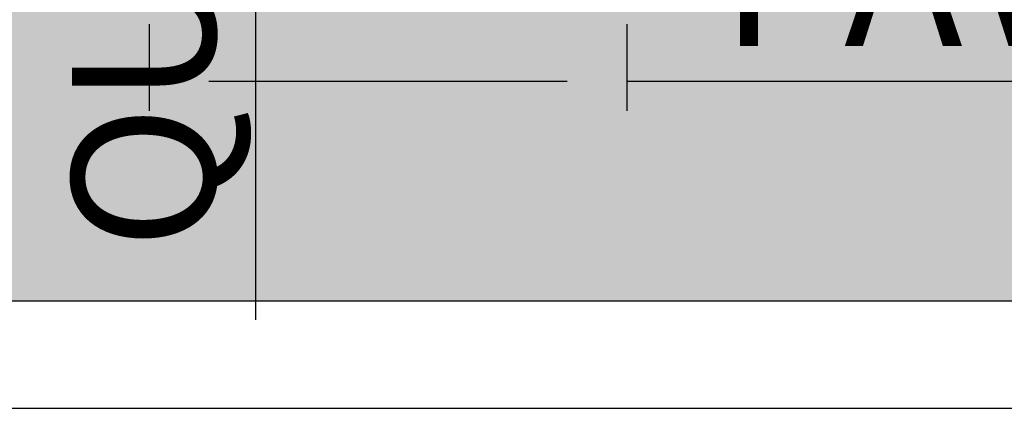
# Model space of a CAD drawing. Units: inches. Extents: x 459864 to 460310, y 324185 to 324787.
# Tile 45 of 112: x 460127 to 460169, y 324195 to 324211. Entities that reach past the tile are written whole.
import ezdxf

# ---------------------------------------------------------------- set-up
doc = ezdxf.new("R2010")
doc.units = ezdxf.units.IN
for name, color, linetype, lineweight in [('A-ANNO-DIMS', 2, 'Continuous', 18), ('C-PROP', 7, 'Continuous', 30), ('L-SITE-PATT', 252, 'Continuous', 13)]:
    doc.layers.add(name, color=color, linetype=linetype, lineweight=lineweight)
doc.styles.get("Standard").update_dxf_attribs({"font": 'arial.ttf'})
doc.dimstyles.new('ISO-25', dxfattribs={"dimtxt": 6, "dimasz": 2.5, "dimexe": 1.25, "dimexo": 0.625, "dimtad": 1, "dimdec": 1, "dimlunit": 3, "dimtxsty": 'Standard', "dimcen": 2.5, "dimadec": 0, "dimazin": 0, "dimtfac": 1, "dimtdec": 1, "dimtmove": 0, "dimatfit": 3, "dimfxl": 1, "dimarcsym": 0})

# ---------------------------------------------------------------- blocks, each defined once
blk = doc.blocks.new('*D28')
at = {"layer": 'A-ANNO-DIMS', "color": 0, "lineweight": -2, "transparency": 16777216}
for p, q in [((460148.65, 324370.7), (460136.025, 324370.7)), ((460137.275, 324368.2), (460137.275, 324293.2)), ((460148.65, 324290.7), (460136.025, 324290.7)), ((460137.275, 324290.7), (460137.275, 324198.69))]:
    blk.add_line(p, q, dxfattribs=at)
at = {"layer": 'A-ANNO-DIMS', "color": 0, "transparency": 16777216}
for points in [[(460136.858, 324368.2), (460137.692, 324368.2), (460137.275, 324370.7)], [(460136.858, 324293.2), (460137.692, 324293.2), (460137.275, 324290.7)]]:
    blk.add_solid(points, dxfattribs=at)
at = {"layer": 'Defpoints', "color": 0, "transparency": 16777216}
for p in [(460149.275, 324370.7), (460137.275, 324290.7), (460149.275, 324290.7)]:
    blk.add_point(p, dxfattribs=at)
at = {"layer": 'A-ANNO-DIMS', "color": 0, "transparency": 16777216, "insert": (460133.363, 324243.445), "char_height": 6, "attachment_point": 5, "rotation": 90}
blk.add_mtext('QUEEN BED 6\'-8" TYP.', dxfattribs=at)
blk = doc.blocks.new('*D34')
at = {"layer": 'A-ANNO-DIMS', "color": 0, "lineweight": -2, "transparency": 16777216}
for p, q in [((460132.814, 324211.063), (460132.814, 324207.434)), ((460152.838, 324211.063), (460152.838, 324207.434)), ((460135.314, 324208.684), (460150.338, 324208.684)), ((460152.838, 324208.684), (460202.984, 324208.684))]:
    blk.add_line(p, q, dxfattribs=at)
at = {"layer": 'A-ANNO-DIMS', "color": 0, "transparency": 16777216}
for points in [[(460135.314, 324209.101), (460135.314, 324208.268), (460132.814, 324208.684)], [(460150.338, 324209.101), (460150.338, 324208.268), (460152.838, 324208.684)]]:
    blk.add_solid(points, dxfattribs=at)
at = {"layer": 'Defpoints', "color": 0, "transparency": 16777216}
for p in [(460132.814, 324211.688), (460152.838, 324211.688), (460152.838, 324208.684)]:
    blk.add_point(p, dxfattribs=at)
at = {"layer": 'A-ANNO-DIMS', "color": 0, "transparency": 16777216, "insert": (460179.161, 324212.373), "char_height": 6, "attachment_point": 5}
blk.add_mtext('PAVER 1\'-8"', dxfattribs=at)

msp = doc.modelspace()

# ---------------------------------------------------------------- hatches: boundary and pattern name
at = {"layer": 'L-SITE-PATT'}
h = msp.add_hatch(dxfattribs=at)
h.set_pattern_fill('DOTS', color=256)
h.paths.add_polyline_path([(460269.804, 324283.483), (460247.115, 324283.483), (460121.929, 324283.483), (460121.929, 324252.473), (460117.429, 324252.473), (460110.124, 324252.473), (460110.124, 324243.287), (460080.83, 324243.287), (460080.83, 324252.473), (460061.115, 324252.473), (460061.115, 324251.882), (460077.909, 324251.882), (460077.909, 324199.483), (460080.83, 324199.483), (460080.83, 324207.553), (460110.124, 324207.553), (460110.124, 324199.483), (460110.813, 324199.483), (460262.115, 324199.483), (460269.804, 324199.483)], flags=17)
edge = h.paths.add_edge_path(flags=0)
edge.add_ellipse((460222.59, 324263.813), major_axis=(-8.485, 8.485), ratio=1, start_angle=405, end_angle=495, ccw=False)
edge.add_line((460214.821, 324254.66), (460214.832, 324254.666))
edge.add_ellipse((460222.59, 324263.813), major_axis=(-8.485, 8.485), ratio=1, start_angle=405, end_angle=495, ccw=False)
edge.add_line((460210.759, 324261.781), (460210.768, 324261.787))
edge.add_ellipse((460222.59, 324263.813), major_axis=(-8.485, 8.485), ratio=1, start_angle=405, end_angle=495, ccw=False)
edge.add_ellipse((460222.59, 324263.813), major_axis=(-8.485, 8.485), ratio=1, start_angle=392.754, end_angle=405, ccw=False)
edge.add_ellipse((460222.59, 324263.813), major_axis=(-8.485, 8.485), ratio=1, start_angle=380.9347, end_angle=392.754, ccw=False)
edge.add_line((460211.337, 324267.985), (460211.34, 324267.985))
edge.add_ellipse((460222.59, 324263.813), major_axis=(-8.485, 8.485), ratio=1, start_angle=380.9347, end_angle=392.754, ccw=False)
edge.add_ellipse((460222.59, 324263.813), major_axis=(-8.485, 8.485), ratio=1, start_angle=347.9015, end_angle=380.9347, ccw=False)
edge.add_ellipse((460222.59, 324263.813), major_axis=(-8.485, 8.485), ratio=1, start_angle=327.0619, end_angle=347.9015, ccw=False)
edge.add_ellipse((460222.59, 324263.813), major_axis=(-8.485, 8.485), ratio=1, start_angle=278.3246, end_angle=327.0619, ccw=False)
edge.add_line((460225.158, 324275.536), (460225.158, 324275.535))
edge.add_ellipse((460222.59, 324263.813), major_axis=(-8.485, 8.485), ratio=1, start_angle=278.3246, end_angle=327.0619, ccw=False)
edge.add_ellipse((460222.59, 324263.813), major_axis=(-8.485, 8.485), ratio=1, start_angle=260.6436, end_angle=278.3246, ccw=False)
edge.add_ellipse((460222.59, 324263.813), major_axis=(-8.485, 8.485), ratio=1, start_angle=225, end_angle=260.6436, ccw=False)
edge.add_line((460234.509, 324265.243), (460234.501, 324265.239))
edge.add_ellipse((460222.59, 324263.813), major_axis=(-8.485, 8.485), ratio=1, start_angle=225, end_angle=260.6436, ccw=False)
edge.add_ellipse((460222.59, 324263.813), major_axis=(-8.485, 8.485), ratio=1, start_angle=495, end_angle=585, ccw=False)
edge.add_line((460234.437, 324261.861), (460234.424, 324261.858))
edge.add_ellipse((460222.59, 324263.813), major_axis=(-8.485, 8.485), ratio=1, start_angle=495, end_angle=585, ccw=False)
edge.add_line((460227.95, 324253.067), (460227.946, 324253.083))
edge.add_ellipse((460222.59, 324263.813), major_axis=(-8.485, 8.485), ratio=1, start_angle=495, end_angle=585, ccw=False)
edge.add_line((460226.223, 324252.369), (460226.211, 324252.38))
edge.add_ellipse((460222.59, 324263.813), major_axis=(-8.485, 8.485), ratio=1, start_angle=495, end_angle=585, ccw=False)
h.paths.add_polyline_path([(460219.651, 324254.347), (460218.461, 324253.545), (460218.275, 324254.789), (460219.642, 324256.542), (460219.625, 324260.848), (460216.11, 324257.333), (460214.35, 324256.978), (460215.416, 324259.356), (460212.524, 324258.496), (460213.137, 324259.93), (460218.507, 324263.813), (460222.59, 324263.813), (460222.59, 324267.807), (460218.176, 324272.212), (460219.026, 324274.639), (460222.59, 324272.811), (460222.59, 324275.423), (460223.057, 324274.825), (460222.675, 324273.492), (460225.912, 324267.135), (460219.625, 324260.848)], flags=0)
edge = h.paths.add_edge_path(flags=0)
edge.add_ellipse((460194.576, 324264.046), major_axis=(-8.485, 8.485), ratio=1, start_angle=495, end_angle=585, ccw=False)
edge.add_line((460199.936, 324253.3), (460199.932, 324253.316))
edge.add_ellipse((460194.576, 324264.046), major_axis=(-8.485, 8.485), ratio=1, start_angle=495, end_angle=585, ccw=False)
edge.add_line((460198.208, 324252.603), (460198.196, 324252.613))
edge.add_ellipse((460194.576, 324264.046), major_axis=(-8.485, 8.485), ratio=1, start_angle=495, end_angle=585, ccw=False)
edge.add_ellipse((460194.576, 324264.046), major_axis=(-8.485, 8.485), ratio=1, start_angle=405, end_angle=495, ccw=False)
edge.add_line((460186.806, 324254.893), (460186.817, 324254.899))
edge.add_ellipse((460194.576, 324264.046), major_axis=(-8.485, 8.485), ratio=1, start_angle=405, end_angle=495, ccw=False)
edge.add_line((460182.744, 324262.014), (460182.753, 324262.02))
edge.add_ellipse((460194.576, 324264.046), major_axis=(-8.485, 8.485), ratio=1, start_angle=405, end_angle=495, ccw=False)
edge.add_ellipse((460194.576, 324264.046), major_axis=(-8.485, 8.485), ratio=1, start_angle=392.754, end_angle=405, ccw=False)
edge.add_ellipse((460194.576, 324264.046), major_axis=(-8.485, 8.485), ratio=1, start_angle=380.9347, end_angle=392.754, ccw=False)
edge.add_line((460183.323, 324268.218), (460183.326, 324268.218))
edge.add_ellipse((460194.576, 324264.046), major_axis=(-8.485, 8.485), ratio=1, start_angle=380.9347, end_angle=392.754, ccw=False)
edge.add_ellipse((460194.576, 324264.046), major_axis=(-8.485, 8.485), ratio=1, start_angle=347.9015, end_angle=380.9347, ccw=False)
edge.add_ellipse((460194.576, 324264.046), major_axis=(-8.485, 8.485), ratio=1, start_angle=327.0619, end_angle=347.9015, ccw=False)
edge.add_ellipse((460194.576, 324264.046), major_axis=(-8.485, 8.485), ratio=1, start_angle=278.3246, end_angle=327.0619, ccw=False)
edge.add_line((460197.144, 324275.769), (460197.143, 324275.768))
edge.add_ellipse((460194.576, 324264.046), major_axis=(-8.485, 8.485), ratio=1, start_angle=278.3246, end_angle=327.0619, ccw=False)
edge.add_ellipse((460194.576, 324264.046), major_axis=(-8.485, 8.485), ratio=1, start_angle=260.6436, end_angle=278.3246, ccw=False)
edge.add_ellipse((460194.576, 324264.046), major_axis=(-8.485, 8.485), ratio=1, start_angle=225, end_angle=260.6436, ccw=False)
edge.add_line((460206.494, 324265.476), (460206.487, 324265.473))
edge.add_ellipse((460194.576, 324264.046), major_axis=(-8.485, 8.485), ratio=1, start_angle=225, end_angle=260.6436, ccw=False)
edge.add_ellipse((460194.576, 324264.046), major_axis=(-8.485, 8.485), ratio=1, start_angle=495, end_angle=585, ccw=False)
edge.add_line((460206.422, 324262.094), (460206.409, 324262.091))
h.paths.add_polyline_path([(460191.61, 324261.081), (460191.637, 324254.58), (460190.447, 324253.778), (460190.261, 324255.023), (460191.628, 324256.775), (460191.61, 324261.081), (460188.096, 324257.566), (460186.335, 324257.211), (460187.402, 324259.589), (460184.509, 324258.729), (460185.123, 324260.163), (460190.493, 324264.046), (460194.576, 324264.046), (460194.576, 324268.04), (460190.161, 324272.446), (460191.011, 324274.872), (460194.576, 324273.044), (460194.576, 324275.657), (460195.043, 324275.058), (460194.661, 324273.725), (460197.897, 324267.368)], flags=0)
edge = h.paths.add_edge_path(flags=0)
edge.add_ellipse((460252.912, 324263.578), major_axis=(-8.485, 8.485), ratio=1, start_angle=405, end_angle=495, ccw=False)
edge.add_line((460241.081, 324261.545), (460241.089, 324261.551))
edge.add_ellipse((460252.912, 324263.578), major_axis=(-8.485, 8.485), ratio=1, start_angle=405, end_angle=495, ccw=False)
edge.add_ellipse((460252.912, 324263.578), major_axis=(-8.485, 8.485), ratio=1, start_angle=392.754, end_angle=405, ccw=False)
edge.add_ellipse((460252.912, 324263.578), major_axis=(-8.485, 8.485), ratio=1, start_angle=380.9347, end_angle=392.754, ccw=False)
edge.add_line((460241.659, 324267.749), (460241.662, 324267.749))
edge.add_ellipse((460252.912, 324263.578), major_axis=(-8.485, 8.485), ratio=1, start_angle=380.9347, end_angle=392.754, ccw=False)
edge.add_ellipse((460252.912, 324263.578), major_axis=(-8.485, 8.485), ratio=1, start_angle=347.9015, end_angle=380.9347, ccw=False)
edge.add_ellipse((460252.912, 324263.578), major_axis=(-8.485, 8.485), ratio=1, start_angle=327.0619, end_angle=347.9015, ccw=False)
edge.add_ellipse((460252.912, 324263.578), major_axis=(-8.485, 8.485), ratio=1, start_angle=278.3246, end_angle=327.0619, ccw=False)
edge.add_line((460255.48, 324275.3), (460255.479, 324275.299))
edge.add_ellipse((460252.912, 324263.578), major_axis=(-8.485, 8.485), ratio=1, start_angle=278.3246, end_angle=327.0619, ccw=False)
edge.add_ellipse((460252.912, 324263.578), major_axis=(-8.485, 8.485), ratio=1, start_angle=260.6436, end_angle=278.3246, ccw=False)
edge.add_ellipse((460252.912, 324263.578), major_axis=(-8.485, 8.485), ratio=1, start_angle=225, end_angle=260.6436, ccw=False)
edge.add_line((460264.83, 324265.007), (460264.823, 324265.004))
edge.add_ellipse((460252.912, 324263.578), major_axis=(-8.485, 8.485), ratio=1, start_angle=225, end_angle=260.6436, ccw=False)
edge.add_ellipse((460252.912, 324263.578), major_axis=(-8.485, 8.485), ratio=1, start_angle=495, end_angle=585, ccw=False)
edge.add_line((460264.758, 324261.626), (460264.745, 324261.622))
edge.add_ellipse((460252.912, 324263.578), major_axis=(-8.485, 8.485), ratio=1, start_angle=495, end_angle=585, ccw=False)
edge.add_line((460258.272, 324252.832), (460258.268, 324252.848))
edge.add_ellipse((460252.912, 324263.578), major_axis=(-8.485, 8.485), ratio=1, start_angle=495, end_angle=585, ccw=False)
edge.add_line((460256.545, 324252.134), (460256.533, 324252.144))
edge.add_ellipse((460252.912, 324263.578), major_axis=(-8.485, 8.485), ratio=1, start_angle=495, end_angle=585, ccw=False)
edge.add_ellipse((460252.912, 324263.578), major_axis=(-8.485, 8.485), ratio=1, start_angle=405, end_angle=495, ccw=False)
edge.add_line((460245.143, 324254.424), (460245.153, 324254.43))
h.paths.add_polyline_path([(460244.672, 324256.742), (460245.738, 324259.12), (460242.846, 324258.26), (460243.459, 324259.694), (460248.829, 324263.578), (460252.912, 324263.578), (460252.912, 324267.571), (460248.497, 324271.977), (460249.348, 324274.403), (460252.912, 324272.576), (460252.912, 324275.188), (460253.379, 324274.589), (460252.997, 324273.257), (460256.233, 324266.899), (460249.946, 324260.612), (460249.973, 324254.111), (460248.783, 324253.309), (460248.597, 324254.554), (460249.964, 324256.306), (460249.946, 324260.612), (460246.432, 324257.097)], flags=0)
edge = h.paths.add_edge_path(flags=0)
edge.add_ellipse((460167.439, 324262.833), major_axis=(-8.485, 8.485), ratio=1, start_angle=495, end_angle=585, ccw=False)
edge.add_line((460172.799, 324252.087), (460172.795, 324252.103))
edge.add_ellipse((460167.439, 324262.833), major_axis=(-8.485, 8.485), ratio=1, start_angle=495, end_angle=585, ccw=False)
edge.add_line((460171.071, 324251.389), (460171.059, 324251.399))
edge.add_ellipse((460167.439, 324262.833), major_axis=(-8.485, 8.485), ratio=1, start_angle=495, end_angle=585, ccw=False)
edge.add_ellipse((460167.439, 324262.833), major_axis=(-8.485, 8.485), ratio=1, start_angle=405, end_angle=495, ccw=False)
edge.add_line((460159.669, 324253.679), (460159.68, 324253.685))
edge.add_ellipse((460167.439, 324262.833), major_axis=(-8.485, 8.485), ratio=1, start_angle=405, end_angle=495, ccw=False)
edge.add_line((460155.607, 324260.8), (460155.616, 324260.806))
edge.add_ellipse((460167.439, 324262.833), major_axis=(-8.485, 8.485), ratio=1, start_angle=405, end_angle=495, ccw=False)
edge.add_ellipse((460167.439, 324262.833), major_axis=(-8.485, 8.485), ratio=1, start_angle=392.754, end_angle=405, ccw=False)
edge.add_ellipse((460167.439, 324262.833), major_axis=(-8.485, 8.485), ratio=1, start_angle=380.9347, end_angle=392.754, ccw=False)
edge.add_line((460156.185, 324267.005), (460156.189, 324267.005))
edge.add_ellipse((460167.439, 324262.833), major_axis=(-8.485, 8.485), ratio=1, start_angle=380.9347, end_angle=392.754, ccw=False)
edge.add_ellipse((460167.439, 324262.833), major_axis=(-8.485, 8.485), ratio=1, start_angle=347.9015, end_angle=380.9347, ccw=False)
edge.add_ellipse((460167.439, 324262.833), major_axis=(-8.485, 8.485), ratio=1, start_angle=327.0619, end_angle=347.9015, ccw=False)
edge.add_ellipse((460167.439, 324262.833), major_axis=(-8.485, 8.485), ratio=1, start_angle=278.3246, end_angle=327.0619, ccw=False)
edge.add_line((460170.007, 324274.556), (460170.006, 324274.554))
edge.add_ellipse((460167.439, 324262.833), major_axis=(-8.485, 8.485), ratio=1, start_angle=278.3246, end_angle=327.0619, ccw=False)
edge.add_ellipse((460167.439, 324262.833), major_axis=(-8.485, 8.485), ratio=1, start_angle=260.6436, end_angle=278.3246, ccw=False)
edge.add_ellipse((460167.439, 324262.833), major_axis=(-8.485, 8.485), ratio=1, start_angle=225, end_angle=260.6436, ccw=False)
edge.add_line((460179.357, 324264.262), (460179.35, 324264.259))
edge.add_ellipse((460167.439, 324262.833), major_axis=(-8.485, 8.485), ratio=1, start_angle=225, end_angle=260.6436, ccw=False)
edge.add_ellipse((460167.439, 324262.833), major_axis=(-8.485, 8.485), ratio=1, start_angle=495, end_angle=585, ccw=False)
edge.add_line((460179.285, 324260.881), (460179.272, 324260.877))
h.paths.add_polyline_path([(460164.473, 324259.867), (460164.5, 324253.366), (460163.31, 324252.565), (460163.124, 324253.809), (460164.491, 324255.561), (460164.473, 324259.867), (460160.958, 324256.353), (460159.198, 324255.998), (460160.265, 324258.375), (460157.372, 324257.515), (460157.986, 324258.949), (460163.356, 324262.833), (460167.439, 324262.833), (460167.439, 324266.826), (460163.024, 324271.232), (460163.874, 324273.659), (460167.439, 324271.831), (460167.439, 324274.443), (460167.905, 324273.844), (460167.524, 324272.512), (460170.76, 324266.154)], flags=0)
edge = h.paths.add_edge_path(flags=0)
edge.add_ellipse((460140.758, 324262.37), major_axis=(-8.485, 8.485), ratio=1, start_angle=495, end_angle=585, ccw=False)
edge.add_line((460146.118, 324251.624), (460146.114, 324251.639))
edge.add_ellipse((460140.758, 324262.37), major_axis=(-8.485, 8.485), ratio=1, start_angle=495, end_angle=585, ccw=False)
edge.add_line((460144.391, 324250.926), (460144.379, 324250.936))
edge.add_ellipse((460140.758, 324262.37), major_axis=(-8.485, 8.485), ratio=1, start_angle=495, end_angle=585, ccw=False)
edge.add_ellipse((460140.758, 324262.37), major_axis=(-8.485, 8.485), ratio=1, start_angle=405, end_angle=495, ccw=False)
edge.add_line((460132.989, 324253.216), (460132.999, 324253.222))
edge.add_ellipse((460140.758, 324262.37), major_axis=(-8.485, 8.485), ratio=1, start_angle=405, end_angle=495, ccw=False)
edge.add_line((460128.927, 324260.337), (460128.935, 324260.343))
edge.add_ellipse((460140.758, 324262.37), major_axis=(-8.485, 8.485), ratio=1, start_angle=405, end_angle=495, ccw=False)
edge.add_ellipse((460140.758, 324262.37), major_axis=(-8.485, 8.485), ratio=1, start_angle=392.754, end_angle=405, ccw=False)
edge.add_ellipse((460140.758, 324262.37), major_axis=(-8.485, 8.485), ratio=1, start_angle=380.9347, end_angle=392.754, ccw=False)
edge.add_line((460129.505, 324266.541), (460129.508, 324266.541))
edge.add_ellipse((460140.758, 324262.37), major_axis=(-8.485, 8.485), ratio=1, start_angle=380.9347, end_angle=392.754, ccw=False)
edge.add_ellipse((460140.758, 324262.37), major_axis=(-8.485, 8.485), ratio=1, start_angle=347.9015, end_angle=380.9347, ccw=False)
edge.add_ellipse((460140.758, 324262.37), major_axis=(-8.485, 8.485), ratio=1, start_angle=327.0619, end_angle=347.9015, ccw=False)
edge.add_ellipse((460140.758, 324262.37), major_axis=(-8.485, 8.485), ratio=1, start_angle=278.3246, end_angle=327.0619, ccw=False)
edge.add_line((460143.326, 324274.092), (460143.325, 324274.091))
edge.add_ellipse((460140.758, 324262.37), major_axis=(-8.485, 8.485), ratio=1, start_angle=278.3246, end_angle=327.0619, ccw=False)
edge.add_ellipse((460140.758, 324262.37), major_axis=(-8.485, 8.485), ratio=1, start_angle=260.6436, end_angle=278.3246, ccw=False)
edge.add_ellipse((460140.758, 324262.37), major_axis=(-8.485, 8.485), ratio=1, start_angle=225, end_angle=260.6436, ccw=False)
edge.add_line((460152.677, 324263.799), (460152.669, 324263.796))
edge.add_ellipse((460140.758, 324262.37), major_axis=(-8.485, 8.485), ratio=1, start_angle=225, end_angle=260.6436, ccw=False)
edge.add_ellipse((460140.758, 324262.37), major_axis=(-8.485, 8.485), ratio=1, start_angle=495, end_angle=585, ccw=False)
edge.add_line((460152.604, 324260.418), (460152.592, 324260.414))
h.paths.add_polyline_path([(460137.792, 324259.404), (460137.819, 324252.903), (460136.629, 324252.101), (460136.443, 324253.346), (460137.81, 324255.098), (460137.792, 324259.404), (460134.278, 324255.889), (460132.518, 324255.534), (460133.584, 324257.912), (460130.692, 324257.052), (460131.305, 324258.486), (460136.675, 324262.37), (460140.758, 324262.37), (460140.758, 324266.363), (460136.343, 324270.769), (460137.194, 324273.195), (460140.758, 324271.367), (460140.758, 324273.98), (460141.225, 324273.381), (460140.843, 324272.049), (460144.079, 324265.691)], flags=0)
h.paths.add_polyline_path([(460110.124, 324227.414), (460080.83, 324227.414), (460080.83, 324235.484), (460110.124, 324235.484)], flags=16)
h.paths.add_polyline_path([(460110.124, 324220.797), (460110.124, 324212.727), (460080.83, 324212.727), (460080.83, 324220.797)], flags=16)
h.paths.add_polyline_path([(460269.804, 324283.483), (460247.115, 324283.483), (460121.929, 324283.483), (460121.929, 324252.473), (460117.429, 324252.473), (460110.124, 324252.473), (460110.124, 324243.287), (460080.83, 324243.287), (460080.83, 324252.473), (460061.115, 324252.473), (460061.115, 324251.882), (460077.909, 324251.882), (460077.909, 324199.483), (460080.83, 324199.483), (460080.83, 324207.553), (460110.124, 324207.553), (460110.124, 324199.483), (460262.115, 324199.483), (460269.804, 324199.483)], flags=17)
h.paths.add_polyline_path([(460219.651, 324254.347), (460218.461, 324253.545), (460218.275, 324254.789), (460219.642, 324256.542), (460219.625, 324260.848), (460216.11, 324257.333), (460214.35, 324256.978), (460215.416, 324259.356), (460212.524, 324258.496), (460213.137, 324259.93), (460218.507, 324263.813), (460222.59, 324263.813), (460220.18, 324266.223), (460215.461, 324265.308), (460211.835, 324266.137), (460216.247, 324267.985), (460218.418, 324267.985), (460222.59, 324263.813), (460222.59, 324267.807), (460218.176, 324272.212), (460219.026, 324274.639), (460222.59, 324272.811), (460222.59, 324275.423), (460223.057, 324274.825), (460222.675, 324273.492), (460225.912, 324267.135), (460222.59, 324263.813), (460231.383, 324263.813), (460228.485, 324262.488), (460224.425, 324261.978), (460228.68, 324257.724), (460228.966, 324254.791), (460227.142, 324256.537), (460227.542, 324254.819), (460227.333, 324253.614), (460222.59, 324259.985), (460222.59, 324255.497), (460221.377, 324256.541), (460220.576, 324261.799), (460219.625, 324260.848)], flags=0)
h.paths.add_polyline_path([(460199.127, 324256.77), (460199.528, 324255.052), (460199.319, 324253.848), (460194.576, 324260.218), (460194.576, 324255.73), (460193.363, 324256.774), (460192.561, 324262.032), (460191.61, 324261.081), (460191.637, 324254.58), (460190.447, 324253.778), (460190.261, 324255.023), (460191.628, 324256.775), (460191.61, 324261.081), (460188.096, 324257.566), (460186.335, 324257.211), (460187.402, 324259.589), (460184.509, 324258.729), (460185.123, 324260.163), (460190.493, 324264.046), (460194.576, 324264.046), (460192.166, 324266.456), (460187.446, 324265.541), (460183.82, 324266.37), (460188.232, 324268.218), (460190.404, 324268.218), (460194.576, 324264.046), (460194.576, 324268.04), (460190.161, 324272.446), (460191.011, 324274.872), (460194.576, 324273.044), (460194.576, 324275.657), (460195.043, 324275.058), (460194.661, 324273.725), (460197.897, 324267.368), (460194.576, 324264.046), (460203.368, 324264.046), (460200.47, 324262.721), (460196.411, 324262.212), (460200.665, 324257.957), (460200.951, 324255.024)], flags=0)
h.paths.add_polyline_path([(460244.672, 324256.742), (460245.738, 324259.12), (460242.846, 324258.26), (460243.459, 324259.694), (460248.829, 324263.578), (460252.912, 324263.578), (460250.502, 324265.987), (460245.783, 324265.072), (460242.156, 324265.901), (460246.568, 324267.749), (460248.74, 324267.749), (460252.912, 324263.578), (460252.912, 324267.571), (460248.497, 324271.977), (460249.348, 324274.403), (460252.912, 324272.576), (460252.912, 324275.188), (460253.379, 324274.589), (460252.997, 324273.257), (460256.233, 324266.899), (460252.912, 324263.578), (460261.705, 324263.578), (460258.806, 324262.252), (460254.747, 324261.743), (460259.002, 324257.488), (460259.288, 324254.555), (460257.463, 324256.301), (460257.864, 324254.583), (460257.655, 324253.379), (460252.912, 324259.749), (460252.912, 324255.261), (460251.699, 324256.305), (460250.897, 324261.563), (460249.946, 324260.612), (460249.973, 324254.111), (460248.783, 324253.309), (460248.597, 324254.554), (460249.964, 324256.306), (460249.946, 324260.612), (460246.432, 324257.097)], flags=0)
h.paths.add_polyline_path([(460173.528, 324256.743), (460173.814, 324253.811), (460171.99, 324255.556), (460172.39, 324253.838), (460172.182, 324252.634), (460167.439, 324259.004), (460167.439, 324254.516), (460166.226, 324255.56), (460165.424, 324260.818), (460164.473, 324259.867), (460164.5, 324253.366), (460163.31, 324252.565), (460163.124, 324253.809), (460164.491, 324255.561), (460164.473, 324259.867), (460160.958, 324256.353), (460159.198, 324255.998), (460160.265, 324258.375), (460157.372, 324257.515), (460157.986, 324258.949), (460163.356, 324262.833), (460167.439, 324262.833), (460165.029, 324265.243), (460160.309, 324264.327), (460156.683, 324265.156), (460161.095, 324267.005), (460163.267, 324267.005), (460167.439, 324262.833), (460167.439, 324266.826), (460163.024, 324271.232), (460163.874, 324273.659), (460167.439, 324271.831), (460167.439, 324274.443), (460167.905, 324273.844), (460167.524, 324272.512), (460170.76, 324266.154), (460167.439, 324262.833), (460176.231, 324262.833), (460173.333, 324261.507), (460169.274, 324260.998)], flags=0)
h.paths.add_polyline_path([(460146.848, 324256.28), (460147.134, 324253.347), (460145.31, 324255.093), (460145.71, 324253.375), (460145.501, 324252.171), (460140.758, 324258.541), (460140.758, 324254.053), (460139.545, 324255.097), (460138.744, 324260.355), (460137.792, 324259.404), (460137.819, 324252.903), (460136.629, 324252.101), (460136.443, 324253.346), (460137.81, 324255.098), (460137.792, 324259.404), (460134.278, 324255.889), (460132.518, 324255.534), (460133.584, 324257.912), (460130.692, 324257.052), (460131.305, 324258.486), (460136.675, 324262.37), (460140.758, 324262.37), (460138.348, 324264.779), (460133.629, 324263.864), (460130.002, 324264.693), (460134.414, 324266.541), (460136.586, 324266.541), (460140.758, 324262.37), (460140.758, 324266.363), (460136.343, 324270.769), (460137.194, 324273.195), (460140.758, 324271.367), (460140.758, 324273.98), (460141.225, 324273.381), (460140.843, 324272.049), (460144.079, 324265.691), (460140.758, 324262.37), (460149.551, 324262.37), (460146.653, 324261.044), (460142.593, 324260.535)], flags=0)
edge = h.paths.add_edge_path()
edge.add_line((460269.804, 324272.549), (460260.881, 324272.549))
edge.add_ellipse((460252.912, 324263.578), major_axis=(-8.485, 8.485), ratio=1, start_angle=260.6436, end_angle=273.3846, ccw=False)
edge.add_line((460262.283, 324271.092), (460262.261, 324271.091))
edge.add_ellipse((460252.912, 324263.578), major_axis=(-8.485, 8.485), ratio=1, start_angle=260.6436, end_angle=273.3846, ccw=False)
edge.add_ellipse((460252.912, 324263.578), major_axis=(-8.485, 8.485), ratio=1, start_angle=225, end_angle=260.6436, ccw=False)
edge.add_line((460263.609, 324269.063), (460263.572, 324269.058))
edge.add_ellipse((460252.912, 324263.578), major_axis=(-8.485, 8.485), ratio=1, start_angle=225, end_angle=260.6436, ccw=False)
edge.add_line((460264.615, 324266.306), (460264.585, 324266.305))
edge.add_ellipse((460252.912, 324263.578), major_axis=(-8.485, 8.485), ratio=1, start_angle=225, end_angle=260.6436, ccw=False)
edge.add_line((460264.83, 324265.007), (460264.823, 324265.004))
edge.add_ellipse((460252.912, 324263.578), major_axis=(-8.485, 8.485), ratio=1, start_angle=225, end_angle=260.6436, ccw=False)
edge.add_ellipse((460252.912, 324263.578), major_axis=(-8.485, 8.485), ratio=1, start_angle=495, end_angle=585, ccw=False)
edge.add_line((460264.758, 324261.626), (460264.745, 324261.622))
edge.add_ellipse((460252.912, 324263.578), major_axis=(-8.485, 8.485), ratio=1, start_angle=495, end_angle=585, ccw=False)
edge.add_line((460263.442, 324257.739), (460263.389, 324257.779))
edge.add_ellipse((460252.912, 324263.578), major_axis=(-8.485, 8.485), ratio=1, start_angle=495, end_angle=585, ccw=False)
edge.add_line((460258.128, 324252.744), (460258.102, 324252.779))
edge.add_ellipse((460252.912, 324263.578), major_axis=(-8.485, 8.485), ratio=1, start_angle=495, end_angle=585, ccw=False)
edge.add_line((460256.545, 324252.134), (460256.533, 324252.144))
edge.add_ellipse((460252.912, 324263.578), major_axis=(-8.485, 8.485), ratio=1, start_angle=495, end_angle=585, ccw=False)
edge.add_ellipse((460252.912, 324263.578), major_axis=(-8.485, 8.485), ratio=1, start_angle=405, end_angle=495, ccw=False)
edge.add_line((460250.594, 324251.78), (460250.605, 324251.82))
edge.add_ellipse((460252.912, 324263.578), major_axis=(-8.485, 8.485), ratio=1, start_angle=405, end_angle=495, ccw=False)
edge.add_line((460245.143, 324254.424), (460245.153, 324254.43))
edge.add_ellipse((460252.912, 324263.578), major_axis=(-8.485, 8.485), ratio=1, start_angle=405, end_angle=495, ccw=False)
edge.add_line((460243.525, 324256.059), (460243.56, 324256.091))
edge.add_ellipse((460252.912, 324263.578), major_axis=(-8.485, 8.485), ratio=1, start_angle=405, end_angle=495, ccw=False)
edge.add_line((460241.44, 324259.893), (460241.522, 324259.896))
edge.add_ellipse((460252.912, 324263.578), major_axis=(-8.485, 8.485), ratio=1, start_angle=405, end_angle=495, ccw=False)
edge.add_line((460241.081, 324261.545), (460241.089, 324261.551))
edge.add_ellipse((460252.912, 324263.578), major_axis=(-8.485, 8.485), ratio=1, start_angle=405, end_angle=495, ccw=False)
edge.add_ellipse((460252.912, 324263.578), major_axis=(-8.485, 8.485), ratio=1, start_angle=392.754, end_angle=405, ccw=False)
edge.add_line((460241.05, 324265.438), (460241.063, 324265.443))
edge.add_ellipse((460252.912, 324263.578), major_axis=(-8.485, 8.485), ratio=1, start_angle=392.754, end_angle=405, ccw=False)
edge.add_ellipse((460252.912, 324263.578), major_axis=(-8.485, 8.485), ratio=1, start_angle=380.9347, end_angle=392.754, ccw=False)
edge.add_line((460241.452, 324267.176), (460241.469, 324267.171))
edge.add_ellipse((460252.912, 324263.578), major_axis=(-8.485, 8.485), ratio=1, start_angle=380.9347, end_angle=392.754, ccw=False)
edge.add_line((460241.659, 324267.749), (460241.662, 324267.749))
edge.add_ellipse((460252.912, 324263.578), major_axis=(-8.485, 8.485), ratio=1, start_angle=380.9347, end_angle=392.754, ccw=False)
edge.add_ellipse((460252.912, 324263.578), major_axis=(-8.485, 8.485), ratio=1, start_angle=356.6154, end_angle=380.9347, ccw=False)
edge.add_line((460244.88, 324272.488), (460244.713, 324272.549))
edge.add_line((460244.713, 324272.549), (460230.817, 324272.549))
edge.add_ellipse((460222.59, 324263.813), major_axis=(-8.485, 8.485), ratio=1, start_angle=260.6436, end_angle=271.7178, ccw=False)
edge.add_ellipse((460222.59, 324263.813), major_axis=(-8.485, 8.485), ratio=1, start_angle=225, end_angle=260.6436, ccw=False)
edge.add_line((460233.287, 324269.299), (460233.25, 324269.294))
edge.add_ellipse((460222.59, 324263.813), major_axis=(-8.485, 8.485), ratio=1, start_angle=225, end_angle=260.6436, ccw=False)
edge.add_line((460234.294, 324266.541), (460234.264, 324266.541))
edge.add_ellipse((460222.59, 324263.813), major_axis=(-8.485, 8.485), ratio=1, start_angle=225, end_angle=260.6436, ccw=False)
edge.add_line((460234.509, 324265.243), (460234.501, 324265.239))
edge.add_ellipse((460222.59, 324263.813), major_axis=(-8.485, 8.485), ratio=1, start_angle=225, end_angle=260.6436, ccw=False)
edge.add_ellipse((460222.59, 324263.813), major_axis=(-8.485, 8.485), ratio=1, start_angle=495, end_angle=585, ccw=False)
edge.add_line((460234.437, 324261.861), (460234.424, 324261.858))
edge.add_ellipse((460222.59, 324263.813), major_axis=(-8.485, 8.485), ratio=1, start_angle=495, end_angle=585, ccw=False)
edge.add_line((460233.121, 324257.975), (460233.068, 324258.015))
edge.add_ellipse((460222.59, 324263.813), major_axis=(-8.485, 8.485), ratio=1, start_angle=495, end_angle=585, ccw=False)
edge.add_line((460227.806, 324252.979), (460227.78, 324253.014))
edge.add_ellipse((460222.59, 324263.813), major_axis=(-8.485, 8.485), ratio=1, start_angle=495, end_angle=585, ccw=False)
edge.add_line((460226.223, 324252.369), (460226.211, 324252.38))
edge.add_ellipse((460222.59, 324263.813), major_axis=(-8.485, 8.485), ratio=1, start_angle=495, end_angle=585, ccw=False)
edge.add_ellipse((460222.59, 324263.813), major_axis=(-8.485, 8.485), ratio=1, start_angle=405, end_angle=495, ccw=False)
edge.add_line((460220.272, 324252.016), (460220.283, 324252.055))
edge.add_ellipse((460222.59, 324263.813), major_axis=(-8.485, 8.485), ratio=1, start_angle=405, end_angle=495, ccw=False)
edge.add_line((460214.821, 324254.66), (460214.832, 324254.666))
edge.add_ellipse((460222.59, 324263.813), major_axis=(-8.485, 8.485), ratio=1, start_angle=405, end_angle=495, ccw=False)
edge.add_line((460213.203, 324256.295), (460213.239, 324256.327))
edge.add_ellipse((460222.59, 324263.813), major_axis=(-8.485, 8.485), ratio=1, start_angle=405, end_angle=495, ccw=False)
edge.add_line((460211.118, 324260.128), (460211.201, 324260.131))
edge.add_ellipse((460222.59, 324263.813), major_axis=(-8.485, 8.485), ratio=1, start_angle=405, end_angle=495, ccw=False)
edge.add_line((460210.759, 324261.781), (460210.768, 324261.787))
edge.add_ellipse((460222.59, 324263.813), major_axis=(-8.485, 8.485), ratio=1, start_angle=405, end_angle=495, ccw=False)
edge.add_ellipse((460222.59, 324263.813), major_axis=(-8.485, 8.485), ratio=1, start_angle=392.754, end_angle=405, ccw=False)
edge.add_line((460210.729, 324265.673), (460210.741, 324265.678))
edge.add_ellipse((460222.59, 324263.813), major_axis=(-8.485, 8.485), ratio=1, start_angle=392.754, end_angle=405, ccw=False)
edge.add_ellipse((460222.59, 324263.813), major_axis=(-8.485, 8.485), ratio=1, start_angle=380.9347, end_angle=392.754, ccw=False)
edge.add_line((460211.13, 324267.412), (460211.147, 324267.407))
edge.add_ellipse((460222.59, 324263.813), major_axis=(-8.485, 8.485), ratio=1, start_angle=380.9347, end_angle=392.754, ccw=False)
edge.add_line((460211.337, 324267.985), (460211.34, 324267.985))
edge.add_ellipse((460222.59, 324263.813), major_axis=(-8.485, 8.485), ratio=1, start_angle=380.9347, end_angle=392.754, ccw=False)
edge.add_ellipse((460222.59, 324263.813), major_axis=(-8.485, 8.485), ratio=1, start_angle=358.2822, end_angle=380.9347, ccw=False)
edge.add_line((460213.705, 324271.902), (460213.709, 324271.869))
edge.add_ellipse((460222.59, 324263.813), major_axis=(-8.485, 8.485), ratio=1, start_angle=358.2822, end_angle=380.9347, ccw=False)
edge.add_line((460214.363, 324272.549), (460203.078, 324272.549))
edge.add_line((460203.078, 324272.549), (460203.06, 324272.531))
edge.add_ellipse((460194.576, 324264.046), major_axis=(-8.485, 8.485), ratio=1, start_angle=260.6436, end_angle=270.1168, ccw=False)
edge.add_line((460203.957, 324271.561), (460203.921, 324271.56))
edge.add_ellipse((460194.576, 324264.046), major_axis=(-8.485, 8.485), ratio=1, start_angle=260.6436, end_angle=270.1168, ccw=False)
edge.add_ellipse((460194.576, 324264.046), major_axis=(-8.485, 8.485), ratio=1, start_angle=225, end_angle=260.6436, ccw=False)
edge.add_line((460205.272, 324269.532), (460205.235, 324269.527))
edge.add_ellipse((460194.576, 324264.046), major_axis=(-8.485, 8.485), ratio=1, start_angle=225, end_angle=260.6436, ccw=False)
edge.add_line((460206.279, 324266.774), (460206.249, 324266.774))
edge.add_ellipse((460194.576, 324264.046), major_axis=(-8.485, 8.485), ratio=1, start_angle=225, end_angle=260.6436, ccw=False)
edge.add_line((460206.494, 324265.476), (460206.487, 324265.473))
edge.add_ellipse((460194.576, 324264.046), major_axis=(-8.485, 8.485), ratio=1, start_angle=225, end_angle=260.6436, ccw=False)
edge.add_ellipse((460194.576, 324264.046), major_axis=(-8.485, 8.485), ratio=1, start_angle=495, end_angle=585, ccw=False)
edge.add_line((460206.422, 324262.094), (460206.409, 324262.091))
edge.add_ellipse((460194.576, 324264.046), major_axis=(-8.485, 8.485), ratio=1, start_angle=495, end_angle=585, ccw=False)
edge.add_line((460205.106, 324258.208), (460205.053, 324258.248))
edge.add_ellipse((460194.576, 324264.046), major_axis=(-8.485, 8.485), ratio=1, start_angle=495, end_angle=585, ccw=False)
edge.add_line((460199.792, 324253.212), (460199.766, 324253.248))
edge.add_ellipse((460194.576, 324264.046), major_axis=(-8.485, 8.485), ratio=1, start_angle=495, end_angle=585, ccw=False)
edge.add_line((460198.208, 324252.603), (460198.196, 324252.613))
edge.add_ellipse((460194.576, 324264.046), major_axis=(-8.485, 8.485), ratio=1, start_angle=495, end_angle=585, ccw=False)
edge.add_ellipse((460194.576, 324264.046), major_axis=(-8.485, 8.485), ratio=1, start_angle=405, end_angle=495, ccw=False)
edge.add_line((460192.258, 324252.249), (460192.268, 324252.289))
edge.add_ellipse((460194.576, 324264.046), major_axis=(-8.485, 8.485), ratio=1, start_angle=405, end_angle=495, ccw=False)
edge.add_line((460186.806, 324254.893), (460186.817, 324254.899))
edge.add_ellipse((460194.576, 324264.046), major_axis=(-8.485, 8.485), ratio=1, start_angle=405, end_angle=495, ccw=False)
edge.add_line((460185.188, 324256.528), (460185.224, 324256.56))
edge.add_ellipse((460194.576, 324264.046), major_axis=(-8.485, 8.485), ratio=1, start_angle=405, end_angle=495, ccw=False)
edge.add_line((460183.104, 324260.362), (460183.186, 324260.365))
edge.add_ellipse((460194.576, 324264.046), major_axis=(-8.485, 8.485), ratio=1, start_angle=405, end_angle=495, ccw=False)
edge.add_line((460182.744, 324262.014), (460182.753, 324262.02))
edge.add_ellipse((460194.576, 324264.046), major_axis=(-8.485, 8.485), ratio=1, start_angle=405, end_angle=495, ccw=False)
edge.add_ellipse((460194.576, 324264.046), major_axis=(-8.485, 8.485), ratio=1, start_angle=392.754, end_angle=405, ccw=False)
edge.add_line((460182.714, 324265.906), (460182.726, 324265.912))
edge.add_ellipse((460194.576, 324264.046), major_axis=(-8.485, 8.485), ratio=1, start_angle=392.754, end_angle=405, ccw=False)
edge.add_ellipse((460194.576, 324264.046), major_axis=(-8.485, 8.485), ratio=1, start_angle=380.9347, end_angle=392.754, ccw=False)
edge.add_line((460183.116, 324267.645), (460183.133, 324267.64))
edge.add_ellipse((460194.576, 324264.046), major_axis=(-8.485, 8.485), ratio=1, start_angle=380.9347, end_angle=392.754, ccw=False)
edge.add_line((460183.323, 324268.218), (460183.326, 324268.218))
edge.add_ellipse((460194.576, 324264.046), major_axis=(-8.485, 8.485), ratio=1, start_angle=380.9347, end_angle=392.754, ccw=False)
edge.add_ellipse((460194.576, 324264.046), major_axis=(-8.485, 8.485), ratio=1, start_angle=359.8832, end_angle=380.9347, ccw=False)
edge.add_line((460184.491, 324270.611), (460184.553, 324270.611))
edge.add_ellipse((460194.576, 324264.046), major_axis=(-8.485, 8.485), ratio=1, start_angle=359.8832, end_angle=380.9347, ccw=False)
edge.add_line((460185.346, 324271.76), (460185.379, 324271.728))
edge.add_ellipse((460194.576, 324264.046), major_axis=(-8.485, 8.485), ratio=1, start_angle=359.8832, end_angle=380.9347, ccw=False)
edge.add_line((460185.697, 324272.086), (460185.633, 324272.549))
edge.add_line((460185.633, 324272.549), (460174.683, 324272.549))
edge.add_line((460174.683, 324272.549), (460174.606, 324272.457))
edge.add_ellipse((460167.439, 324262.833), major_axis=(-8.485, 8.485), ratio=1, start_angle=260.6436, end_angle=278.3246, ccw=False)
edge.add_ellipse((460167.439, 324262.833), major_axis=(-8.485, 8.485), ratio=1, start_angle=225, end_angle=260.6436, ccw=False)
edge.add_line((460178.135, 324268.318), (460178.098, 324268.313))
edge.add_ellipse((460167.439, 324262.833), major_axis=(-8.485, 8.485), ratio=1, start_angle=225, end_angle=260.6436, ccw=False)
edge.add_line((460179.142, 324265.561), (460179.112, 324265.56))
edge.add_ellipse((460167.439, 324262.833), major_axis=(-8.485, 8.485), ratio=1, start_angle=225, end_angle=260.6436, ccw=False)
edge.add_line((460179.357, 324264.262), (460179.35, 324264.259))
edge.add_ellipse((460167.439, 324262.833), major_axis=(-8.485, 8.485), ratio=1, start_angle=225, end_angle=260.6436, ccw=False)
edge.add_ellipse((460167.439, 324262.833), major_axis=(-8.485, 8.485), ratio=1, start_angle=495, end_angle=585, ccw=False)
edge.add_line((460179.285, 324260.881), (460179.272, 324260.877))
edge.add_ellipse((460167.439, 324262.833), major_axis=(-8.485, 8.485), ratio=1, start_angle=495, end_angle=585, ccw=False)
edge.add_line((460177.969, 324256.994), (460177.916, 324257.034))
edge.add_ellipse((460167.439, 324262.833), major_axis=(-8.485, 8.485), ratio=1, start_angle=495, end_angle=585, ccw=False)
edge.add_line((460172.655, 324251.999), (460172.629, 324252.034))
edge.add_ellipse((460167.439, 324262.833), major_axis=(-8.485, 8.485), ratio=1, start_angle=495, end_angle=585, ccw=False)
edge.add_line((460171.071, 324251.389), (460171.059, 324251.399))
edge.add_ellipse((460167.439, 324262.833), major_axis=(-8.485, 8.485), ratio=1, start_angle=495, end_angle=585, ccw=False)
edge.add_ellipse((460167.439, 324262.833), major_axis=(-8.485, 8.485), ratio=1, start_angle=405, end_angle=495, ccw=False)
edge.add_line((460165.121, 324251.036), (460165.131, 324251.075))
edge.add_ellipse((460167.439, 324262.833), major_axis=(-8.485, 8.485), ratio=1, start_angle=405, end_angle=495, ccw=False)
edge.add_line((460159.669, 324253.679), (460159.68, 324253.685))
edge.add_ellipse((460167.439, 324262.833), major_axis=(-8.485, 8.485), ratio=1, start_angle=405, end_angle=495, ccw=False)
edge.add_line((460158.051, 324255.314), (460158.087, 324255.347))
edge.add_ellipse((460167.439, 324262.833), major_axis=(-8.485, 8.485), ratio=1, start_angle=405, end_angle=495, ccw=False)
edge.add_line((460155.967, 324259.148), (460156.049, 324259.151))
edge.add_ellipse((460167.439, 324262.833), major_axis=(-8.485, 8.485), ratio=1, start_angle=405, end_angle=495, ccw=False)
edge.add_line((460155.607, 324260.8), (460155.616, 324260.806))
edge.add_ellipse((460167.439, 324262.833), major_axis=(-8.485, 8.485), ratio=1, start_angle=405, end_angle=495, ccw=False)
edge.add_ellipse((460167.439, 324262.833), major_axis=(-8.485, 8.485), ratio=1, start_angle=392.754, end_angle=405, ccw=False)
edge.add_line((460155.577, 324264.693), (460155.589, 324264.698))
edge.add_ellipse((460167.439, 324262.833), major_axis=(-8.485, 8.485), ratio=1, start_angle=392.754, end_angle=405, ccw=False)
edge.add_ellipse((460167.439, 324262.833), major_axis=(-8.485, 8.485), ratio=1, start_angle=380.9347, end_angle=392.754, ccw=False)
edge.add_line((460155.979, 324266.432), (460155.996, 324266.426))
edge.add_ellipse((460167.439, 324262.833), major_axis=(-8.485, 8.485), ratio=1, start_angle=380.9347, end_angle=392.754, ccw=False)
edge.add_line((460156.185, 324267.005), (460156.189, 324267.005))
edge.add_ellipse((460167.439, 324262.833), major_axis=(-8.485, 8.485), ratio=1, start_angle=380.9347, end_angle=392.754, ccw=False)
edge.add_ellipse((460167.439, 324262.833), major_axis=(-8.485, 8.485), ratio=1, start_angle=350.9345, end_angle=380.9347, ccw=False)
edge.add_line((460157.363, 324269.397), (460157.414, 324269.397))
edge.add_ellipse((460167.439, 324262.833), major_axis=(-8.485, 8.485), ratio=1, start_angle=350.9345, end_angle=380.9347, ccw=False)
edge.add_line((460158.221, 324270.535), (460158.236, 324270.519))
edge.add_ellipse((460167.439, 324262.833), major_axis=(-8.485, 8.485), ratio=1, start_angle=350.9345, end_angle=380.9347, ccw=False)
edge.add_line((460159.379, 324271.753), (460159.419, 324271.738))
edge.add_ellipse((460167.439, 324262.833), major_axis=(-8.485, 8.485), ratio=1, start_angle=350.9345, end_angle=380.9347, ccw=False)
edge.add_line((460160.396, 324272.549), (460147.112, 324272.549))
edge.add_ellipse((460140.758, 324262.37), major_axis=(-8.485, 8.485), ratio=1, start_angle=278.3246, end_angle=283.0261, ccw=False)
edge.add_ellipse((460140.758, 324262.37), major_axis=(-8.485, 8.485), ratio=1, start_angle=260.6436, end_angle=278.3246, ccw=False)
edge.add_ellipse((460140.758, 324262.37), major_axis=(-8.485, 8.485), ratio=1, start_angle=225, end_angle=260.6436, ccw=False)
edge.add_line((460151.455, 324267.855), (460151.418, 324267.85))
edge.add_ellipse((460140.758, 324262.37), major_axis=(-8.485, 8.485), ratio=1, start_angle=225, end_angle=260.6436, ccw=False)
edge.add_line((460152.462, 324265.098), (460152.431, 324265.097))
edge.add_ellipse((460140.758, 324262.37), major_axis=(-8.485, 8.485), ratio=1, start_angle=225, end_angle=260.6436, ccw=False)
edge.add_line((460152.677, 324263.799), (460152.669, 324263.796))
edge.add_ellipse((460140.758, 324262.37), major_axis=(-8.485, 8.485), ratio=1, start_angle=225, end_angle=260.6436, ccw=False)
edge.add_ellipse((460140.758, 324262.37), major_axis=(-8.485, 8.485), ratio=1, start_angle=495, end_angle=585, ccw=False)
edge.add_line((460152.604, 324260.418), (460152.592, 324260.414))
edge.add_ellipse((460140.758, 324262.37), major_axis=(-8.485, 8.485), ratio=1, start_angle=495, end_angle=585, ccw=False)
edge.add_line((460151.288, 324256.531), (460151.235, 324256.571))
edge.add_ellipse((460140.758, 324262.37), major_axis=(-8.485, 8.485), ratio=1, start_angle=495, end_angle=585, ccw=False)
edge.add_line((460145.974, 324251.535), (460145.948, 324251.571))
edge.add_ellipse((460140.758, 324262.37), major_axis=(-8.485, 8.485), ratio=1, start_angle=495, end_angle=585, ccw=False)
edge.add_line((460144.391, 324250.926), (460144.379, 324250.936))
edge.add_ellipse((460140.758, 324262.37), major_axis=(-8.485, 8.485), ratio=1, start_angle=495, end_angle=585, ccw=False)
edge.add_ellipse((460140.758, 324262.37), major_axis=(-8.485, 8.485), ratio=1, start_angle=405, end_angle=495, ccw=False)
edge.add_line((460138.44, 324250.572), (460138.451, 324250.612))
edge.add_ellipse((460140.758, 324262.37), major_axis=(-8.485, 8.485), ratio=1, start_angle=405, end_angle=495, ccw=False)
edge.add_line((460132.989, 324253.216), (460132.999, 324253.222))
edge.add_ellipse((460140.758, 324262.37), major_axis=(-8.485, 8.485), ratio=1, start_angle=405, end_angle=495, ccw=False)
edge.add_line((460131.371, 324254.851), (460131.406, 324254.883))
edge.add_ellipse((460140.758, 324262.37), major_axis=(-8.485, 8.485), ratio=1, start_angle=405, end_angle=495, ccw=False)
edge.add_line((460129.286, 324258.685), (460129.369, 324258.688))
edge.add_ellipse((460140.758, 324262.37), major_axis=(-8.485, 8.485), ratio=1, start_angle=405, end_angle=495, ccw=False)
edge.add_line((460128.927, 324260.337), (460128.935, 324260.343))
edge.add_ellipse((460140.758, 324262.37), major_axis=(-8.485, 8.485), ratio=1, start_angle=405, end_angle=495, ccw=False)
edge.add_ellipse((460140.758, 324262.37), major_axis=(-8.485, 8.485), ratio=1, start_angle=392.754, end_angle=405, ccw=False)
edge.add_line((460128.896, 324264.23), (460128.909, 324264.235))
edge.add_ellipse((460140.758, 324262.37), major_axis=(-8.485, 8.485), ratio=1, start_angle=392.754, end_angle=405, ccw=False)
edge.add_ellipse((460140.758, 324262.37), major_axis=(-8.485, 8.485), ratio=1, start_angle=380.9347, end_angle=392.754, ccw=False)
edge.add_line((460129.298, 324265.968), (460129.315, 324265.963))
edge.add_ellipse((460140.758, 324262.37), major_axis=(-8.485, 8.485), ratio=1, start_angle=380.9347, end_angle=392.754, ccw=False)
edge.add_line((460129.505, 324266.541), (460129.508, 324266.541))
edge.add_ellipse((460140.758, 324262.37), major_axis=(-8.485, 8.485), ratio=1, start_angle=380.9347, end_angle=392.754, ccw=False)
edge.add_ellipse((460140.758, 324262.37), major_axis=(-8.485, 8.485), ratio=1, start_angle=347.9015, end_angle=380.9347, ccw=False)
edge.add_line((460130.697, 324268.934), (460130.727, 324268.934))
edge.add_ellipse((460140.758, 324262.37), major_axis=(-8.485, 8.485), ratio=1, start_angle=347.9015, end_angle=380.9347, ccw=False)
edge.add_line((460131.869, 324270.48), (460131.879, 324270.413))
edge.add_ellipse((460140.758, 324262.37), major_axis=(-8.485, 8.485), ratio=1, start_angle=347.9015, end_angle=380.9347, ccw=False)
edge.add_line((460132.734, 324271.277), (460132.705, 324271.287))
edge.add_ellipse((460140.758, 324262.37), major_axis=(-8.485, 8.485), ratio=1, start_angle=347.9015, end_angle=380.9347, ccw=False)
edge.add_line((460134.24, 324272.445), (460134.204, 324272.549))
edge.add_line((460134.204, 324272.549), (460121.929, 324272.549))
edge.add_line((460121.929, 324272.549), (460121.929, 324252.473))
edge.add_line((460121.929, 324252.473), (460117.429, 324252.473))
edge.add_line((460117.429, 324252.473), (460110.124, 324252.473))
edge.add_line((460110.124, 324252.473), (460110.124, 324243.287))
edge.add_line((460110.124, 324243.287), (460080.83, 324243.287))
edge.add_line((460080.83, 324243.287), (460080.83, 324252.473))
edge.add_line((460080.83, 324252.473), (460061.115, 324252.473))
edge.add_line((460061.115, 324252.473), (460061.115, 324251.882))
edge.add_line((460061.115, 324251.882), (460077.909, 324251.882))
edge.add_line((460077.909, 324251.882), (460077.909, 324199.483))
edge.add_line((460077.909, 324199.483), (460080.83, 324199.483))
edge.add_line((460080.83, 324199.483), (460080.83, 324207.553))
edge.add_line((460080.83, 324207.553), (460110.124, 324207.553))
edge.add_line((460110.124, 324207.553), (460110.124, 324199.483))
edge.add_line((460110.124, 324199.483), (460110.813, 324199.483))
edge.add_line((460110.813, 324199.483), (460262.115, 324199.483))
edge.add_line((460262.115, 324199.483), (460269.804, 324199.483))
edge.add_line((460269.804, 324199.483), (460269.804, 324272.549))

# ---------------------------------------------------------------- linework, layer by layer
at = {"layer": 'C-PROP'}
for p, q in [((460061.115, 324199.483), (460262.115, 324199.483)), ((460061.115, 324194.983), (460271.115, 324194.983))]:
    msp.add_line(p, q, dxfattribs=at)

# ---------------------------------------------------------------- dimensions: what is measured, and where the dimension line sits
at = {"layer": 'A-ANNO-DIMS'}
dim = msp.add_linear_dim(base=(460137.275, 324290.7), p1=(460149.275, 324370.7), p2=(460149.275, 324290.7), angle=270, text='QUEEN BED <> TYP.', dimstyle='ISO-25', override={"dimdec": 1, "dimlfac": 1, "dimrnd": 0, "dimzin": 1, "dimdsep": 46, "dimlunit": 4, "dimfrac": 2}, dxfattribs=at)
dim.commit()
dim.dimension.update_dxf_attribs({"geometry": '*D28', "text_midpoint": (460133.363, 324243.445)})
dim = msp.add_linear_dim(base=(460152.838, 324208.684), p1=(460132.814, 324211.688), p2=(460152.838, 324211.688), text='PAVER <>', dimstyle='ISO-25', override={"dimdec": 1, "dimlfac": 1, "dimrnd": 0, "dimzin": 1, "dimdsep": 46, "dimlunit": 4, "dimfrac": 2}, dxfattribs=at)
dim.commit()
dim.dimension.update_dxf_attribs({"geometry": '*D34', "text_midpoint": (460179.161, 324212.373)})

doc.saveas('drawing.dxf')
